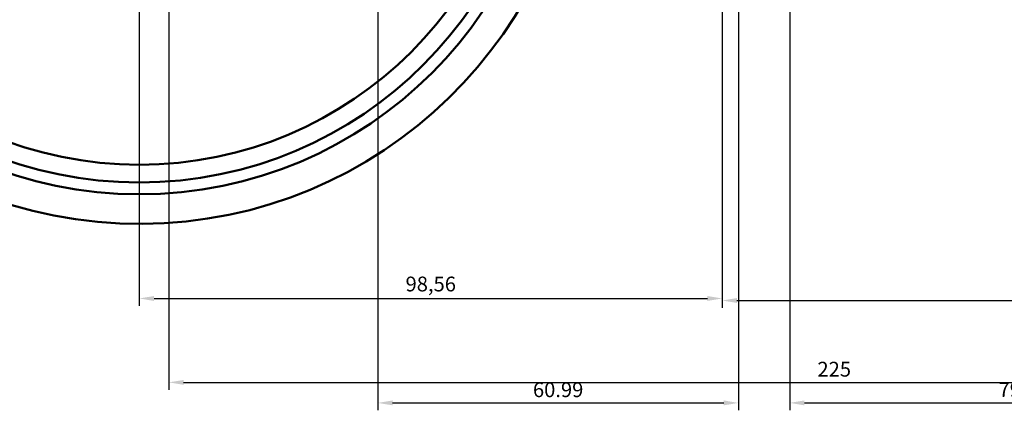
# Model space of a CAD drawing. Units: millimetres. Extents: x 1068 to 1546, y 1743 to 2032.
# Tile 2 of 9: x 1152 to 1318, y 1743 to 1809. Entities that reach past the tile are written whole.
import ezdxf

# ---------------------------------------------------------------- set-up
doc = ezdxf.new("R2010")
doc.units = ezdxf.units.MM
doc.layers.add('M-DIMS', color=2, linetype='Continuous', lineweight=25)
doc.layers.add('M-OUTL', color=7, linetype='Continuous', lineweight=50)
doc.styles.get("Standard").update_dxf_attribs({"font": 'arial.ttf'})
doc.dimstyles.new('ISO-25', dxfattribs={"dimtxt": 2.5, "dimasz": 2.5, "dimexe": 1.25, "dimexo": 0.625, "dimtad": 1, "dimtxsty": 'Standard', "dimcen": 2.5, "dimadec": 0, "dimazin": 0, "dimtfac": 1, "dimtmove": 0, "dimatfit": 3, "dimfxl": 1, "dimarcsym": 0})

# ---------------------------------------------------------------- blocks, each defined once
blk = doc.blocks.new('*D5')
at = {"layer": 'Defpoints', "color": 0, "transparency": 16777216}
for p in [(1177.23, 1849.76), (1402.23, 1849.76), (1402.23, 1747.98)]:
    blk.add_point(p, dxfattribs=at)
at = {"layer": 'M-DIMS', "color": 0, "lineweight": -2, "transparency": 16777216}
for p, q in [((1177.23, 1849.14), (1177.23, 1746.73)), ((1402.23, 1849.14), (1402.23, 1746.73)), ((1179.73, 1747.98), (1399.73, 1747.98))]:
    blk.add_line(p, q, dxfattribs=at)
at = {"layer": 'M-DIMS', "color": 0, "transparency": 16777216}
for points in [[(1179.73, 1748.39), (1179.73, 1747.56), (1177.23, 1747.98)], [(1399.73, 1748.39), (1399.73, 1747.56), (1402.23, 1747.98)]]:
    blk.add_solid(points, dxfattribs=at)
at = {"layer": 'M-DIMS', "color": 0, "transparency": 16777216, "insert": (1289.73, 1749.88), "char_height": 2.5, "attachment_point": 5}
blk.add_mtext('225', dxfattribs=at)
blk = doc.blocks.new('*D6')
at = {"layer": 'Defpoints', "color": 0, "transparency": 16777216}
for p in [(1172.23, 1849.76), (1270.79, 1849.76), (1270.79, 1762.16)]:
    blk.add_point(p, dxfattribs=at)
at = {"layer": 'M-DIMS', "color": 0, "lineweight": -2, "transparency": 16777216}
for p, q in [((1172.23, 1849.14), (1172.23, 1760.91)), ((1270.79, 1849.14), (1270.79, 1760.91)), ((1174.73, 1762.16), (1268.29, 1762.16))]:
    blk.add_line(p, q, dxfattribs=at)
at = {"layer": 'M-DIMS', "color": 0, "transparency": 16777216}
for points in [[(1174.73, 1762.57), (1174.73, 1761.74), (1172.23, 1762.16)], [(1268.29, 1762.57), (1268.29, 1761.74), (1270.79, 1762.16)]]:
    blk.add_solid(points, dxfattribs=at)
at = {"layer": 'M-DIMS', "color": 0, "transparency": 16777216, "insert": (1221.51, 1764.28), "char_height": 2.5, "attachment_point": 5}
blk.add_mtext('98,56', dxfattribs=at)
blk = doc.blocks.new('*D12')
at = {"layer": 'Defpoints', "color": 0, "transparency": 16777216}
for p in [(1172.23, 1849.76), (1169.46, 1845.6)]:
    blk.add_point(p, dxfattribs=at)
at = {"layer": 'M-DIMS', "color": 0, "lineweight": -2, "transparency": 16777216}
for p, q in [((1172.23, 1849.76), (1169.46, 1845.6)), ((1115.28, 1764.16), (1168.07, 1843.52))]:
    blk.add_line(p, q, dxfattribs=at)
at = {"layer": 'M-DIMS', "color": 0, "transparency": 16777216}
blk.add_solid([(1167.73, 1843.75), (1168.42, 1843.29), (1169.46, 1845.6)], dxfattribs=at)
at = {"layer": 'M-DIMS', "color": 0, "transparency": 16777216, "insert": (1115.17, 1767.42), "char_height": 2.5, "attachment_point": 5, "rotation": 56.3651}
blk.add_mtext('R5', dxfattribs=at)
blk = doc.blocks.new('*D13')
at = {"layer": 'Defpoints', "color": 0, "transparency": 16777216}
for p in [(1172.23, 1849.76), (1161.59, 1839.19)]:
    blk.add_point(p, dxfattribs=at)
at = {"layer": 'M-DIMS', "color": 0, "lineweight": -2, "transparency": 16777216}
for p, q in [((1172.23, 1849.76), (1161.59, 1839.19)), ((1102.29, 1780.3), (1159.81, 1837.43))]:
    blk.add_line(p, q, dxfattribs=at)
at = {"layer": 'M-DIMS', "color": 0, "transparency": 16777216}
blk.add_solid([(1159.52, 1837.73), (1160.11, 1837.13), (1161.59, 1839.19)], dxfattribs=at)
at = {"layer": 'M-DIMS', "color": 0, "transparency": 16777216, "insert": (1103.52, 1784.2), "char_height": 2.5, "attachment_point": 5, "rotation": 44.8055}
blk.add_mtext('R15', dxfattribs=at)
blk = doc.blocks.new('*D14')
at = {"layer": 'Defpoints', "color": 0, "transparency": 16777216}
for p in [(1172.23, 1849.76), (1116.4, 1816.48)]:
    blk.add_point(p, dxfattribs=at)
at = {"layer": 'M-DIMS', "color": 0, "lineweight": -2, "transparency": 16777216}
for p, q in [((1172.23, 1849.76), (1116.4, 1816.48)), ((1080.65, 1795.17), (1114.25, 1815.2))]:
    blk.add_line(p, q, dxfattribs=at)
at = {"layer": 'M-DIMS', "color": 0, "transparency": 16777216}
blk.add_solid([(1114.03, 1815.56), (1114.46, 1814.84), (1116.4, 1816.48)], dxfattribs=at)
at = {"layer": 'M-DIMS', "color": 0, "transparency": 16777216, "insert": (1082.79, 1798.66), "char_height": 2.5, "attachment_point": 5, "rotation": 30.7992}
blk.add_mtext('R65', dxfattribs=at)
blk = doc.blocks.new('*D24')
at = {"layer": 'Defpoints', "color": 0, "transparency": 16777216}
for p in [(1270.79, 1850.31), (1402.23, 1850.31), (1402.23, 1761.81)]:
    blk.add_point(p, dxfattribs=at)
at = {"layer": 'M-DIMS', "color": 0, "lineweight": -2, "transparency": 16777216}
for p, q in [((1270.79, 1849.68), (1270.79, 1760.56)), ((1402.23, 1849.68), (1402.23, 1760.56)), ((1273.29, 1761.81), (1399.73, 1761.81))]:
    blk.add_line(p, q, dxfattribs=at)
at = {"layer": 'M-DIMS', "color": 0, "transparency": 16777216}
for points in [[(1273.29, 1762.23), (1273.29, 1761.4), (1270.79, 1761.81)], [(1399.73, 1762.23), (1399.73, 1761.4), (1402.23, 1761.81)]]:
    blk.add_solid(points, dxfattribs=at)
at = {"layer": 'M-DIMS', "color": 0, "transparency": 16777216, "insert": (1336.51, 1763.94), "char_height": 2.5, "attachment_point": 5}
blk.add_mtext('131,44', dxfattribs=at)
blk = doc.blocks.new('*D45')
at = {"layer": 'Defpoints', "color": 0, "transparency": 16777216}
for p in [(1212.56, 1957.56), (1273.55, 1860.03), (1273.55, 1744.51)]:
    blk.add_point(p, dxfattribs=at)
at = {"layer": 'M-DIMS', "color": 0, "lineweight": -2, "transparency": 16777216}
for p, q in [((1212.56, 1956.94), (1212.56, 1743.26)), ((1273.55, 1859.4), (1273.55, 1743.26)), ((1215.06, 1744.51), (1271.05, 1744.51))]:
    blk.add_line(p, q, dxfattribs=at)
at = {"layer": 'M-DIMS', "color": 0, "transparency": 16777216}
for points in [[(1215.06, 1744.93), (1215.06, 1744.1), (1212.56, 1744.51)], [(1271.05, 1744.93), (1271.05, 1744.1), (1273.55, 1744.51)]]:
    blk.add_solid(points, dxfattribs=at)
at = {"layer": 'M-DIMS', "color": 0, "transparency": 16777216, "insert": (1243.05, 1746.41), "char_height": 2.5, "attachment_point": 5}
blk.add_mtext('60.99', dxfattribs=at)
blk = doc.blocks.new('*D47')
at = {"layer": 'Defpoints', "color": 0, "transparency": 16777216}
for p in [(1361.34, 1946.14), (1282.2, 1868.65), (1361.34, 1744.51)]:
    blk.add_point(p, dxfattribs=at)
at = {"layer": 'M-DIMS', "color": 0, "lineweight": -2, "transparency": 16777216}
for p, q in [((1361.34, 1945.51), (1361.34, 1743.26)), ((1282.2, 1868.03), (1282.2, 1743.26)), ((1284.7, 1744.51), (1358.84, 1744.51))]:
    blk.add_line(p, q, dxfattribs=at)
at = {"layer": 'M-DIMS', "color": 0, "transparency": 16777216}
for points in [[(1284.7, 1744.93), (1284.7, 1744.1), (1282.2, 1744.51)], [(1358.84, 1744.93), (1358.84, 1744.1), (1361.34, 1744.51)]]:
    blk.add_solid(points, dxfattribs=at)
at = {"layer": 'M-DIMS', "color": 0, "transparency": 16777216, "insert": (1321.77, 1746.41), "char_height": 2.5, "attachment_point": 5}
blk.add_mtext('79.14', dxfattribs=at)

msp = doc.modelspace()

# ---------------------------------------------------------------- linework, layer by layer
at = {"layer": 'M-OUTL'}
for radius in [70, 68, 65]:
    msp.add_circle((1172.2281, 1849.7623), radius, dxfattribs=at)
msp.add_arc((1172.2281, 1849.7623), 75, 2.898254, 355.67622, dxfattribs=at)

# ---------------------------------------------------------------- dimensions: what is measured, and where the dimension line sits
at = {"layer": 'M-DIMS'}
for base, p1, p2, override, picture, middle in [((1273.5484, 1744.5123), (1212.5594, 1957.5607), (1273.5484, 1860.0259), {"dimdec": 2, "dimlfac": 1, "dimrnd": 0, "dimzin": 0, "dimdsep": 46, "dimlunit": 2}, '*D45', (1243.0539, 1746.4138)), ((1361.339, 1744.5123), (1282.1954, 1868.6519), (1361.339, 1946.1377), {"dimdec": 2, "dimlfac": 1, "dimrnd": 0, "dimzin": 0, "dimdsep": 46, "dimlunit": 2}, '*D47', (1321.7672, 1746.4138)), ((1270.787, 1762.1558), (1172.2281, 1849.7623), (1270.787, 1849.7623), {"dimclrd": 0, "dimclre": 0, "dimclrt": 0}, '*D6', (1221.5076, 1764.2832)), ((1402.2281, 1747.9766), (1177.2281, 1849.7623), (1402.2281, 1849.7623), {"dimclrd": 0, "dimclre": 0, "dimclrt": 0}, '*D5', (1289.7281, 1749.8781)), ((1402.2281, 1761.8125), (1270.787, 1850.3085), (1402.2281, 1850.3085), {"dimclrd": 0, "dimclre": 0, "dimclrt": 0}, '*D24', (1336.5076, 1763.9399))]:
    dim = msp.add_linear_dim(base=base, p1=p1, p2=p2, dimstyle='ISO-25', override=override, dxfattribs=at)
    dim.commit()
    dim.dimension.update_dxf_attribs({"geometry": picture, "text_midpoint": middle})
for mpoint, picture, middle in [((1116.3952, 1816.4804), '*D14', (1083.764, 1797.0289)), ((1161.5856, 1839.1918), '*D13', (1104.8597, 1782.8497)), ((1169.4586, 1845.5994), '*D12', (1116.7499, 1766.3712))]:
    dim = msp.add_radius_dim(center=(1172.2281, 1849.7623), mpoint=mpoint, dimstyle='ISO-25', override={"dimclrd": 0, "dimclre": 0, "dimclrt": 0}, dxfattribs=at)
    dim.commit()
    dim.dimension.update_dxf_attribs({"geometry": picture, "text_midpoint": middle, "dimtype": 164})

doc.saveas('drawing.dxf')
